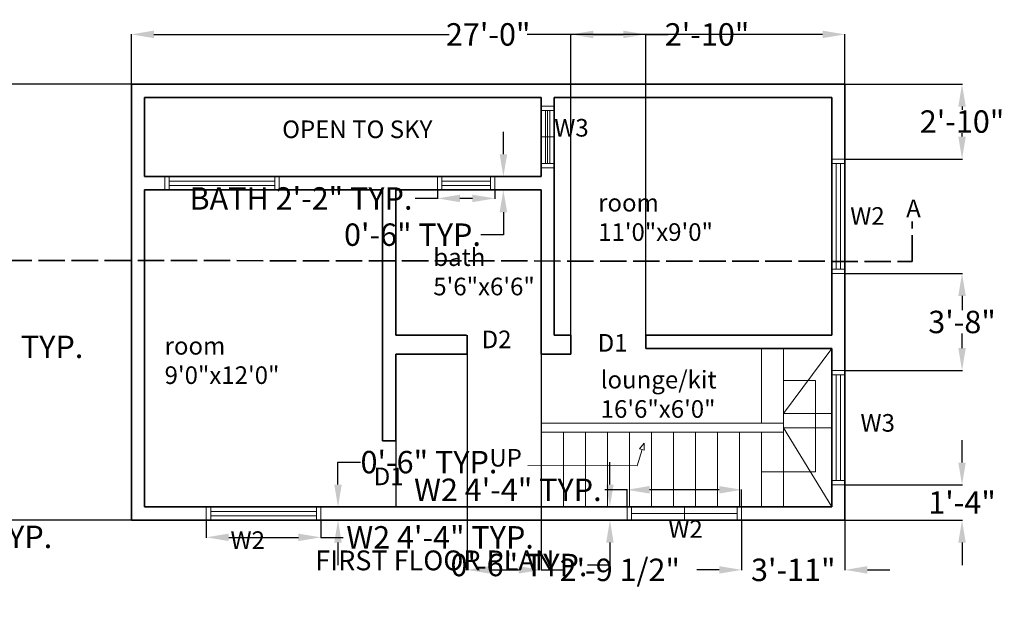
# Model space of a CAD drawing. Units: inches. Extents: x 2393 to 3270, y 740 to 1442.
# Tile 4 of 5: x 2823 to 3270, y 753 to 1018. Entities that reach past the tile are written whole.
import ezdxf

# ---------------------------------------------------------------- set-up
doc = ezdxf.new("R2010")
doc.units = ezdxf.units.IN
doc.header["$MEASUREMENT"] = 0
doc.linetypes.add('ACAD_ISO02W100', pattern=[15, 12, -3])
for name, color, linetype, lineweight in [('A-ANNO-DIMS', 2, 'Continuous', 18), ('A-ANNO-SECT', 1, 'ACAD_ISO02W100', 35), ('A-ANNO-SYMB', 3, 'Continuous', 18), ('A-ANNO-TEXT', 7, 'Continuous', 18), ('A-ANNO-TITL', 7, 'Continuous', 25), ('A-AREA-IDEN', 7, 'Continuous', 18), ('A-DOOR', 3, 'Continuous', 25), ('A-FLOR-STRS', 6, 'Continuous', 18), ('A-GLAZ', 4, 'Continuous', 18), ('A-WALL', 7, 'Continuous', 35)]:
    doc.layers.add(name, color=color, linetype=linetype, lineweight=lineweight)
doc.styles.get("Standard").update_dxf_attribs({"font": 'arial.ttf'})
doc.dimstyles.get("Standard").update_dxf_attribs({"dimtxt": 10.18, "dimasz": 10.18, "dimexe": 0.18, "dimexo": 0.0625, "dimgap": 0.09, "dimtad": 0, "dimtih": 1, "dimtoh": 1, "dimdec": 0, "dimzin": 0, "dimdsep": 46, "dimlunit": 3, "dimtxsty": 'Standard', "dimcen": 0.09, "dimadec": 0, "dimazin": 0, "dimtfac": 1, "dimtdec": 0, "dimtofl": 0, "dimtmove": 0, "dimatfit": 3, "dimfxl": 1, "dimtolj": 1, "dimtzin": 0, "dimarcsym": 0})

# ---------------------------------------------------------------- blocks, each defined once
blk = doc.blocks.new('WIN-52-PLAN')
for p, q in [((0, 6), (0, 0)), ((2, 6), (2, 0)), ((50, 6), (50, 0)), ((52, 6), (52, 0)), ((2, 4), (50, 4)), ((2, 2), (50, 2))]:
    blk.add_line(p, q)
blk = doc.blocks.new('WIN-26-BATH-PLAN')
for p, q in [((0, 0), (0, 6)), ((2, 0), (2, 6)), ((24, 0), (24, 6)), ((26, 0), (26, 6)), ((2, 4), (24, 4)), ((2, 2), (24, 2))]:
    blk.add_line(p, q)
blk = doc.blocks.new('WIN-W3-SIDE-PLAN')
for p, q in [((0, 52), (6, 52)), ((0, 50), (6, 50)), ((2, 50), (2, 2)), ((4, 50), (4, 2)), ((4, 50), (4, 2)), ((4, 50), (4, 2)), ((0, 2), (6, 2)), ((0, 0), (6, 0))]:
    blk.add_line(p, q)
blk = doc.blocks.new('WIN-W2-MULLION-PLAN')
for p, q in [((0, 6), (0, 0)), ((2, 6), (2, 0)), ((26, 6), (26, 0)), ((50, 6), (50, 0)), ((52, 6), (52, 0)), ((2, 3), (50, 3))]:
    blk.add_line(p, q)
blk = doc.blocks.new('WIN-W2-FRONT-PLAN')
for p, q in [((0, 6), (0, 0)), ((2, 6), (2, 0)), ((50, 6), (50, 0)), ((50, 6), (50, 0)), ((52, 6), (52, 0)), ((2, 4), (50, 4)), ((2, 2), (50, 2))]:
    blk.add_line(p, q)
blk = doc.blocks.new('WIN-W3-COURT-PLAN')
for p, q in [((0, 28), (6, 28)), ((0, 26), (6, 26)), ((2, 26), (2, 2)), ((3, 26), (3, 2)), ((4, 26), (4, 2)), ((0, 14), (6, 14)), ((0, 2), (6, 2)), ((0, 0), (6, 0))]:
    blk.add_line(p, q)
blk = doc.blocks.new('STAIR-FLIGHT-PLAN')
for p, q in [((100, 72), (100, 38)), ((100, 72), (100, 38)), ((100, 72), (100, 38)), ((110, 72), (110, 0)), ((110, 72), (110, 0)), ((110, 72), (110, 0)), ((0, 38), (0, 0)), ((110, 38), (0, 38)), ((110, 34), (0, 34)), ((10, 34), (10, 0)), ((20, 34), (20, 0)), ((30, 34), (30, 0)), ((30, 34), (30, 0)), ((30, 34), (30, 0)), ((40, 34), (40, 0)), ((50, 34), (50, 0)), ((60, 34), (60, 0)), ((70, 34), (70, 0)), ((80, 34), (80, 0)), ((80, 34), (80, 0)), ((90, 34), (90, 0)), ((100, 34), (100, 0)), ((100, 34), (100, 0)), ((100, 34), (100, 0))]:
    blk.add_line(p, q)
blk = doc.blocks.new('*D25')
at = {"layer": 'A-ANNO-DIMS', "color": 0, "lineweight": -2, "transparency": 16777216}
for p, q in [((2749.27, 790.69), (2749.27, 782.77)), ((2755.27, 790.69), (2755.27, 782.77)), ((2739.09, 782.95), (2728.91, 782.95)), ((2765.45, 782.95), (2775.63, 782.95))]:
    blk.add_line(p, q, dxfattribs=at)
at = {"layer": 'A-ANNO-DIMS', "color": 0, "transparency": 16777216}
for points in [[(2739.09, 784.65), (2739.09, 781.26), (2749.27, 782.95)], [(2765.45, 784.65), (2765.45, 781.26), (2755.27, 782.95)]]:
    blk.add_solid(points, dxfattribs=at)
at = {"layer": 'Defpoints', "color": 0, "transparency": 16777216}
for p in [(2749.27, 790.75), (2755.27, 790.75), (2755.27, 782.95)]:
    blk.add_point(p, dxfattribs=at)
at = {"layer": 'A-ANNO-DIMS', "color": 0, "transparency": 16777216, "insert": (2806.75, 782.95), "char_height": 10.18, "attachment_point": 5}
blk.add_mtext('\\A1;0\'-6" TYP.', dxfattribs=at)
blk = doc.blocks.new('*D26')
at = {"layer": 'A-ANNO-DIMS', "color": 0, "lineweight": -2, "transparency": 16777216}
for p, q in [((3098.85, 804.33), (3088.67, 804.33)), ((3098.85, 796.6), (3098.85, 804.51)), ((3140.67, 804.33), (3109.03, 804.33)), ((3150.85, 796.6), (3150.85, 804.51))]:
    blk.add_line(p, q, dxfattribs=at)
at = {"layer": 'A-ANNO-DIMS', "color": 0, "transparency": 16777216}
for points in [[(3109.03, 806.03), (3109.03, 802.64), (3098.85, 804.33)], [(3140.67, 806.03), (3140.67, 802.64), (3150.85, 804.33)]]:
    blk.add_solid(points, dxfattribs=at)
at = {"layer": 'Defpoints', "color": 0, "transparency": 16777216}
for p in [(3098.85, 804.33), (3098.85, 796.53), (3150.85, 796.53)]:
    blk.add_point(p, dxfattribs=at)
at = {"layer": 'A-ANNO-DIMS', "color": 0, "transparency": 16777216, "insert": (3044.7, 804.33), "char_height": 10.18, "attachment_point": 5}
blk.add_mtext('\\A1;W2 4\'-4" TYP.', dxfattribs=at)
blk = doc.blocks.new('*D27')
at = {"layer": 'A-ANNO-DIMS', "color": 0, "lineweight": -2, "transparency": 16777216}
for p, q in [((3091.05, 806.71), (3091.05, 816.89)), ((3098.78, 796.53), (3090.87, 796.53)), ((3098.78, 790.53), (3090.87, 790.53)), ((3091.05, 780.35), (3091.05, 770.17)), ((3091.05, 770.17), (3080.87, 770.17))]:
    blk.add_line(p, q, dxfattribs=at)
at = {"layer": 'A-ANNO-DIMS', "color": 0, "transparency": 16777216}
for points in [[(3089.35, 806.71), (3092.74, 806.71), (3091.05, 796.53)], [(3089.35, 780.35), (3092.74, 780.35), (3091.05, 790.53)]]:
    blk.add_solid(points, dxfattribs=at)
at = {"layer": 'Defpoints', "color": 0, "transparency": 16777216}
for p in [(3098.85, 796.53), (3091.05, 790.53), (3098.85, 790.53)]:
    blk.add_point(p, dxfattribs=at)
at = {"layer": 'A-ANNO-DIMS', "color": 0, "transparency": 16777216, "insert": (3049.75, 770.17), "char_height": 10.18, "attachment_point": 5}
blk.add_mtext('\\A1;0\'-6" TYP.', dxfattribs=at)
blk = doc.blocks.new('*D28')
at = {"layer": 'A-ANNO-DIMS', "color": 0, "lineweight": -2, "transparency": 16777216}
for p, q in [((3012.78, 940.47), (3012.78, 936.45)), ((3038.78, 940.47), (3038.78, 936.45)), ((3012.78, 936.63), (3002.6, 936.63)), ((3028.6, 936.63), (3022.96, 936.63))]:
    blk.add_line(p, q, dxfattribs=at)
at = {"layer": 'A-ANNO-DIMS', "color": 0, "transparency": 16777216}
for points in [[(3022.96, 938.33), (3022.96, 934.94), (3012.78, 936.63)], [(3028.6, 938.33), (3028.6, 934.94), (3038.78, 936.63)]]:
    blk.add_solid(points, dxfattribs=at)
at = {"layer": 'Defpoints', "color": 0, "transparency": 16777216}
for p in [(3012.78, 940.53), (3038.78, 940.53), (3012.78, 936.63)]:
    blk.add_point(p, dxfattribs=at)
at = {"layer": 'A-ANNO-DIMS', "color": 0, "transparency": 16777216, "insert": (2950.77, 936.63), "char_height": 10.18, "attachment_point": 5}
blk.add_mtext('\\A1;BATH 2\'-2" TYP.', dxfattribs=at)
blk = doc.blocks.new('*D29')
at = {"layer": 'A-ANNO-DIMS', "color": 0, "lineweight": -2, "transparency": 16777216}
for p, q in [((3042.68, 956.71), (3042.68, 966.89)), ((3038.84, 946.53), (3042.86, 946.53)), ((3038.84, 940.53), (3042.86, 940.53)), ((3042.68, 930.35), (3042.68, 920.17)), ((3042.68, 920.17), (3032.5, 920.17))]:
    blk.add_line(p, q, dxfattribs=at)
at = {"layer": 'A-ANNO-DIMS', "color": 0, "transparency": 16777216}
for points in [[(3040.98, 956.71), (3044.38, 956.71), (3042.68, 946.53)], [(3040.98, 930.35), (3044.38, 930.35), (3042.68, 940.53)]]:
    blk.add_solid(points, dxfattribs=at)
at = {"layer": 'Defpoints', "color": 0, "transparency": 16777216}
for p in [(3038.78, 946.53), (3038.78, 940.53), (3042.68, 940.53)]:
    blk.add_point(p, dxfattribs=at)
at = {"layer": 'A-ANNO-DIMS', "color": 0, "transparency": 16777216, "insert": (3001.39, 920.17), "char_height": 10.18, "attachment_point": 5}
blk.add_mtext('\\A1;0\'-6" TYP.', dxfattribs=at)
blk = doc.blocks.new('*D30')
at = {"layer": 'A-ANNO-DIMS', "color": 0, "lineweight": -2, "transparency": 16777216}
for p, q in [((2907.78, 790.47), (2907.78, 782.55)), ((2959.78, 790.47), (2959.78, 782.55)), ((2917.96, 782.73), (2949.6, 782.73)), ((2959.78, 782.73), (2969.96, 782.73))]:
    blk.add_line(p, q, dxfattribs=at)
at = {"layer": 'A-ANNO-DIMS', "color": 0, "transparency": 16777216}
for points in [[(2917.96, 784.43), (2917.96, 781.04), (2907.78, 782.73)], [(2949.6, 784.43), (2949.6, 781.04), (2959.78, 782.73)]]:
    blk.add_solid(points, dxfattribs=at)
at = {"layer": 'Defpoints', "color": 0, "transparency": 16777216}
for p in [(2907.78, 790.53), (2959.78, 790.53), (2959.78, 782.73)]:
    blk.add_point(p, dxfattribs=at)
at = {"layer": 'A-ANNO-DIMS', "color": 0, "transparency": 16777216, "insert": (3013.93, 782.73), "char_height": 10.18, "attachment_point": 5}
blk.add_mtext('\\A1;W2 4\'-4" TYP.', dxfattribs=at)
blk = doc.blocks.new('*D31')
at = {"layer": 'A-ANNO-DIMS', "color": 0, "lineweight": -2, "transparency": 16777216}
for p, q in [((2967.58, 806.71), (2967.58, 816.89)), ((2967.58, 816.89), (2977.76, 816.89)), ((2959.84, 796.53), (2967.76, 796.53)), ((2959.84, 790.53), (2967.76, 790.53)), ((2967.58, 780.35), (2967.58, 770.17))]:
    blk.add_line(p, q, dxfattribs=at)
at = {"layer": 'A-ANNO-DIMS', "color": 0, "transparency": 16777216}
for points in [[(2965.88, 806.71), (2969.28, 806.71), (2967.58, 796.53)], [(2965.88, 780.35), (2969.28, 780.35), (2967.58, 790.53)]]:
    blk.add_solid(points, dxfattribs=at)
at = {"layer": 'Defpoints', "color": 0, "transparency": 16777216}
for p in [(2959.78, 796.53), (2967.58, 796.53), (2959.78, 790.53)]:
    blk.add_point(p, dxfattribs=at)
at = {"layer": 'A-ANNO-DIMS', "color": 0, "transparency": 16777216, "insert": (3008.88, 816.89), "char_height": 10.18, "attachment_point": 5}
blk.add_mtext('\\A1;0\'-6" TYP.', dxfattribs=at)
blk = doc.blocks.new('*D34')
at = {"layer": 'A-ANNO-DIMS', "color": 0, "lineweight": -2, "transparency": 16777216}
for p, q in [((2617.41, 852.81), (2617.41, 869.43)), ((2627.59, 869.25), (2717.23, 869.25)), ((2727.41, 852.81), (2727.41, 869.43)), ((2727.41, 869.25), (2737.59, 869.25))]:
    blk.add_line(p, q, dxfattribs=at)
at = {"layer": 'A-ANNO-DIMS', "color": 0, "transparency": 16777216}
for points in [[(2627.59, 870.95), (2627.59, 867.56), (2617.41, 869.25)], [(2717.23, 870.95), (2717.23, 867.56), (2727.41, 869.25)]]:
    blk.add_solid(points, dxfattribs=at)
at = {"layer": 'Defpoints', "color": 0, "transparency": 16777216}
for p in [(2727.41, 869.25), (2617.41, 852.75), (2727.41, 852.75)]:
    blk.add_point(p, dxfattribs=at)
at = {"layer": 'A-ANNO-DIMS', "color": 0, "transparency": 16777216, "insert": (2795.67, 869.25), "char_height": 10.18, "attachment_point": 5}
blk.add_mtext('\\A1;FLIGHT 9\'-2" TYP.', dxfattribs=at)
blk = doc.blocks.new('*D49')
at = {"layer": 'A-ANNO-DIMS', "color": 0, "lineweight": -2, "transparency": 16777216}
for p, q in [((3250.94, 816.71), (3250.94, 826.89)), ((3197.84, 806.53), (3251.12, 806.53)), ((3197.84, 790.53), (3251.12, 790.53)), ((3250.94, 780.35), (3250.94, 770.17))]:
    blk.add_line(p, q, dxfattribs=at)
at = {"layer": 'A-ANNO-DIMS', "color": 0, "transparency": 16777216}
for points in [[(3249.24, 816.71), (3252.64, 816.71), (3250.94, 806.53)], [(3249.24, 780.35), (3252.64, 780.35), (3250.94, 790.53)]]:
    blk.add_solid(points, dxfattribs=at)
at = {"layer": 'Defpoints', "color": 0, "transparency": 16777216}
for p in [(3197.78, 806.53), (3250.94, 806.53), (3197.78, 790.53)]:
    blk.add_point(p, dxfattribs=at)
at = {"layer": 'A-ANNO-DIMS', "color": 0, "transparency": 16777216, "insert": (3250.94, 798.53), "char_height": 10.18, "attachment_point": 5}
blk.add_mtext('\\A1;1\'-4"', dxfattribs=at)
blk = doc.blocks.new('*D50')
at = {"layer": 'A-ANNO-DIMS', "color": 0, "lineweight": -2, "transparency": 16777216}
for p, q in [((3197.84, 902.53), (3251.12, 902.53)), ((3250.94, 892.35), (3250.94, 885.83)), ((3250.94, 868.71), (3250.94, 875.24)), ((3197.84, 858.53), (3251.12, 858.53))]:
    blk.add_line(p, q, dxfattribs=at)
at = {"layer": 'A-ANNO-DIMS', "color": 0, "transparency": 16777216}
for points in [[(3249.24, 892.35), (3252.64, 892.35), (3250.94, 902.53)], [(3249.24, 868.71), (3252.64, 868.71), (3250.94, 858.53)]]:
    blk.add_solid(points, dxfattribs=at)
at = {"layer": 'Defpoints', "color": 0, "transparency": 16777216}
for p in [(3197.78, 902.53), (3250.94, 902.53), (3197.78, 858.53)]:
    blk.add_point(p, dxfattribs=at)
at = {"layer": 'A-ANNO-DIMS', "color": 0, "transparency": 16777216, "insert": (3250.94, 880.53), "char_height": 10.18, "attachment_point": 5}
blk.add_mtext('\\A1;3\'-8"', dxfattribs=at)
blk = doc.blocks.new('*D51')
at = {"layer": 'A-ANNO-DIMS', "color": 0, "lineweight": -2, "transparency": 16777216}
for p, q in [((3197.84, 988.53), (3251.12, 988.53)), ((3250.94, 978.35), (3250.94, 976.82)), ((3250.94, 964.71), (3250.94, 966.25)), ((3197.84, 954.53), (3251.12, 954.53))]:
    blk.add_line(p, q, dxfattribs=at)
at = {"layer": 'A-ANNO-DIMS', "color": 0, "transparency": 16777216}
for points in [[(3249.24, 978.35), (3252.64, 978.35), (3250.94, 988.53)], [(3249.24, 964.71), (3252.64, 964.71), (3250.94, 954.53)]]:
    blk.add_solid(points, dxfattribs=at)
at = {"layer": 'Defpoints', "color": 0, "transparency": 16777216}
for p in [(3197.78, 988.53), (3250.94, 988.53), (3197.78, 954.53)]:
    blk.add_point(p, dxfattribs=at)
at = {"layer": 'A-ANNO-DIMS', "color": 0, "transparency": 16777216, "insert": (3250.94, 971.53), "char_height": 10.18, "attachment_point": 5}
blk.add_mtext('\\A1;2\'-10"', dxfattribs=at)
blk = doc.blocks.new('*D52')
at = {"layer": 'A-ANNO-DIMS', "color": 0, "lineweight": -2, "transparency": 16777216}
for p, q in [((3150.85, 790.47), (3150.85, 767.78)), ((3197.78, 790.47), (3197.78, 767.78)), ((3140.67, 767.96), (3130.49, 767.96)), ((3207.96, 767.96), (3218.14, 767.96))]:
    blk.add_line(p, q, dxfattribs=at)
at = {"layer": 'A-ANNO-DIMS', "color": 0, "transparency": 16777216}
for points in [[(3140.67, 769.66), (3140.67, 766.26), (3150.85, 767.96)], [(3207.96, 769.66), (3207.96, 766.26), (3197.78, 767.96)]]:
    blk.add_solid(points, dxfattribs=at)
at = {"layer": 'Defpoints', "color": 0, "transparency": 16777216}
for p in [(3150.85, 790.53), (3197.78, 790.53), (3197.78, 767.96)]:
    blk.add_point(p, dxfattribs=at)
at = {"layer": 'A-ANNO-DIMS', "color": 0, "transparency": 16777216, "insert": (3174.31, 767.96), "char_height": 10.18, "attachment_point": 5}
blk.add_mtext('\\A1;3\'-11"', dxfattribs=at)
blk = doc.blocks.new('*D53')
at = {"layer": 'A-ANNO-DIMS', "color": 0, "lineweight": -2, "transparency": 16777216}
for p, q in [((2873.78, 988.6), (2873.78, 1011.29)), ((2883.96, 1011.11), (3018.12, 1011.11)), ((3187.6, 1011.11), (3053.44, 1011.11)), ((3197.78, 988.6), (3197.78, 1011.29))]:
    blk.add_line(p, q, dxfattribs=at)
at = {"layer": 'A-ANNO-DIMS', "color": 0, "transparency": 16777216}
for points in [[(2883.96, 1012.81), (2883.96, 1009.41), (2873.78, 1011.11)], [(3187.6, 1012.81), (3187.6, 1009.41), (3197.78, 1011.11)]]:
    blk.add_solid(points, dxfattribs=at)
at = {"layer": 'Defpoints', "color": 0, "transparency": 16777216}
for p in [(3197.78, 1011.11), (2873.78, 988.53), (3197.78, 988.53)]:
    blk.add_point(p, dxfattribs=at)
at = {"layer": 'A-ANNO-DIMS', "color": 0, "transparency": 16777216, "insert": (3035.78, 1011.11), "char_height": 10.18, "attachment_point": 5}
blk.add_mtext('\\A1;27\'-0"', dxfattribs=at)
blk = doc.blocks.new('*D54')
at = {"layer": 'A-ANNO-DIMS', "color": 0, "lineweight": -2, "transparency": 16777216}
for p, q in [((2873.72, 988.53), (2763.87, 988.53)), ((2764.05, 978.35), (2764.05, 894.82)), ((2764.05, 800.71), (2764.05, 884.25)), ((2873.72, 790.53), (2763.87, 790.53))]:
    blk.add_line(p, q, dxfattribs=at)
at = {"layer": 'A-ANNO-DIMS', "color": 0, "transparency": 16777216}
for points in [[(2762.35, 978.35), (2765.75, 978.35), (2764.05, 988.53)], [(2762.35, 800.71), (2765.75, 800.71), (2764.05, 790.53)]]:
    blk.add_solid(points, dxfattribs=at)
at = {"layer": 'Defpoints', "color": 0, "transparency": 16777216}
for p in [(2764.05, 988.53), (2873.78, 988.53), (2873.78, 790.53)]:
    blk.add_point(p, dxfattribs=at)
at = {"layer": 'A-ANNO-DIMS', "color": 0, "transparency": 16777216, "insert": (2764.05, 889.53), "char_height": 10.18, "attachment_point": 5}
blk.add_mtext('\\A1;16\'-6"', dxfattribs=at)
blk = doc.blocks.new('*D55')
at = {"layer": 'A-ANNO-DIMS', "color": 0, "lineweight": -2, "transparency": 16777216}
for p, q in [((3026.23, 865.83), (3026.23, 767.78)), ((3059.78, 865.83), (3059.78, 767.78)), ((3036.41, 767.96), (3049.6, 767.96)), ((3059.78, 767.96), (3069.96, 767.96))]:
    blk.add_line(p, q, dxfattribs=at)
at = {"layer": 'A-ANNO-DIMS', "color": 0, "transparency": 16777216}
for points in [[(3036.41, 769.66), (3036.41, 766.26), (3026.23, 767.96)], [(3049.6, 769.66), (3049.6, 766.26), (3059.78, 767.96)]]:
    blk.add_solid(points, dxfattribs=at)
at = {"layer": 'Defpoints', "color": 0, "transparency": 16777216}
for p in [(3026.23, 865.89), (3059.78, 865.89), (3059.78, 767.96)]:
    blk.add_point(p, dxfattribs=at)
at = {"layer": 'A-ANNO-DIMS', "color": 0, "transparency": 16777216, "insert": (3095.53, 767.96), "char_height": 10.18, "attachment_point": 5}
blk.add_mtext('\\A1;2\'-9 1/2"', dxfattribs=at)
blk = doc.blocks.new('*D56')
at = {"layer": 'A-ANNO-DIMS', "color": 0, "lineweight": -2, "transparency": 16777216}
for p, q in [((3073.35, 874.6), (3073.35, 1011.29)), ((3083.53, 1011.11), (3097.13, 1011.11)), ((3107.31, 874.6), (3107.31, 1011.29)), ((3107.31, 1011.11), (3117.49, 1011.11))]:
    blk.add_line(p, q, dxfattribs=at)
at = {"layer": 'A-ANNO-DIMS', "color": 0, "transparency": 16777216}
for points in [[(3083.53, 1012.81), (3083.53, 1009.41), (3073.35, 1011.11)], [(3097.13, 1012.81), (3097.13, 1009.41), (3107.31, 1011.11)]]:
    blk.add_solid(points, dxfattribs=at)
at = {"layer": 'Defpoints', "color": 0, "transparency": 16777216}
for p in [(3107.31, 1011.11), (3073.35, 874.53), (3107.31, 874.53)]:
    blk.add_point(p, dxfattribs=at)
at = {"layer": 'A-ANNO-DIMS', "color": 0, "transparency": 16777216, "insert": (3135.15, 1011.11), "char_height": 10.18, "attachment_point": 5}
blk.add_mtext('\\A1;2\'-10"', dxfattribs=at)

msp = doc.modelspace()

# ---------------------------------------------------------------- linework, layer by layer
at = {"layer": 'A-ANNO-SECT'}
for p, q in [((3228.37, 908.02), (3228.37, 926.08)), ((2786.62, 908.53), (3228.37, 908.02))]:
    msp.add_line(p, q, dxfattribs=at)
at = {"layer": 'A-ANNO-SYMB'}
for p, q in [((3106.64, 825.49), (3104.48, 822.93)), ((3105.75, 822.55), (3104.48, 822.93)), ((3104.48, 822.93), (3106.64, 822.28)), ((3106.64, 822.28), (3106.64, 825.49)), ((3103.48, 815.13), (3105.75, 822.55)), ((3053.71, 815.38), (3103.48, 815.13))]:
    msp.add_line(p, q, dxfattribs=at)
at = {"layer": 'A-DOOR'}
msp.add_line((2993.78, 826.53), (2993.78, 796.53), dxfattribs=at)
at = {"layer": 'A-FLOR-STRS'}
for p, q in [((3169.92, 838.97), (3191.78, 868.53)), ((3169.92, 853.88), (3169.92, 853.88)), ((3169.92, 853.88), (3184.39, 853.88)), ((3184.39, 853.88), (3184.39, 812.49)), ((3169.92, 838.97), (3191.78, 838.97)), ((3169.92, 832.53), (3191.78, 832.53)), ((3169.92, 832.53), (3191.78, 796.53)), ((3184.39, 812.49), (3159.92, 812.49))]:
    msp.add_line(p, q, dxfattribs=at)
at = {"layer": 'A-WALL'}
for p, q in [((2873.78, 790.53), (2873.78, 988.53)), ((2873.78, 988.53), (3197.78, 988.53)), ((3197.78, 988.53), (3197.78, 790.53)), ((2879.78, 946.53), (2879.78, 982.53)), ((2879.78, 982.53), (2987.78, 982.53)), ((2987.78, 982.53), (2993.78, 982.53)), ((2993.78, 982.53), (3059.78, 982.53)), ((3059.78, 946.53), (3059.78, 982.53)), ((3065.78, 874.53), (3065.78, 982.53)), ((3065.78, 982.53), (3191.78, 982.53)), ((3191.78, 982.53), (3191.78, 874.53)), ((2987.78, 946.53), (2879.78, 946.53)), ((2993.78, 946.53), (2987.78, 946.53)), ((3059.78, 946.53), (2993.78, 946.53)), ((2879.78, 862.53), (2879.78, 940.53)), ((2987.78, 940.53), (2879.78, 940.53)), ((2987.78, 862.53), (2987.78, 940.53)), ((2993.78, 874.53), (2993.78, 940.53)), ((3059.78, 940.53), (2993.78, 940.53)), ((3059.78, 940.53), (3059.78, 865.89)), ((2993.78, 874.53), (3025.95, 874.53)), ((3026.23, 865.89), (3026.23, 874.53)), ((3065.78, 874.53), (3073.35, 874.53)), ((3073.35, 874.53), (3073.35, 868.53)), ((3107.31, 874.53), (3191.78, 874.53)), ((3107.31, 874.53), (3107.31, 868.53)), ((3073.35, 865.89), (3073.35, 868.53)), ((3107.31, 868.53), (3191.78, 868.53)), ((3191.78, 868.53), (3191.78, 796.53)), ((2993.78, 862.53), (2993.78, 865.89)), ((2993.78, 865.89), (3026.23, 865.89)), ((3059.78, 865.89), (3065.78, 865.89)), ((3065.78, 865.89), (3073.35, 865.89)), ((2879.78, 856.53), (2879.78, 862.53)), ((2987.78, 856.53), (2987.78, 862.53)), ((2993.78, 862.53), (2993.78, 856.53)), ((2879.78, 796.53), (2879.78, 856.53)), ((2987.78, 826.53), (2987.78, 856.53)), ((2993.78, 826.53), (2993.78, 856.53)), ((2987.78, 826.53), (2993.78, 826.53)), ((2987.78, 796.53), (2879.78, 796.53)), ((2987.78, 796.53), (2993.78, 796.53)), ((3011.44, 796.53), (2993.78, 796.53)), ((3011.44, 796.53), (3057.91, 796.53)), ((3191.78, 796.53), (3057.91, 796.53)), ((3011.44, 790.53), (2873.78, 790.53)), ((3011.44, 790.53), (3057.91, 790.53)), ((3197.78, 790.53), (3057.91, 790.53))]:
    msp.add_line(p, q, dxfattribs=at)

# ---------------------------------------------------------------- block references
at = {"layer": 'A-FLOR-STRS'}
msp.add_blockref('STAIR-FLIGHT-PLAN', (3059.92, 796.53), dxfattribs=at)
at = {"layer": 'A-GLAZ'}
for name, p, rotation in [('WIN-W3-COURT-PLAN', (3065.78, 978.53), 180), ('WIN-52-PLAN', (3191.78, 954.53), 269.9999999999983), ('WIN-52-PLAN', (2940.92, 946.53), 180), ('WIN-26-BATH-PLAN', (3038.78, 946.53), 180), ('WIN-W2-MULLION-PLAN', (3150.85, 796.53), 180)]:
    msp.add_blockref(name, p, dxfattribs=dict(at, rotation=rotation))
for name, p in [('WIN-W3-SIDE-PLAN', (3191.78, 806.53)), ('WIN-W2-FRONT-PLAN', (2907.78, 790.53))]:
    msp.add_blockref(name, p, dxfattribs=at)

# ---------------------------------------------------------------- texts
at = {"layer": 'A-ANNO-SYMB', "char_height": 8, "attachment_point": 1}
for s, insert in [('A', (3225.57, 936.1)), ('UP', (3036.3, 822.87))]:
    msp.add_mtext_dynamic_manual_height_columns(s, width=76.737, gutter_width=1, heights=[0], dxfattribs=dict(at, insert=insert))
at = {"layer": 'A-ANNO-TEXT', "char_height": 8, "attachment_point": 1}
for s, insert in [('W3', (3065.78, 972.71)), ('W2', (3200.17, 932.66)), ('D2', (3032.8, 876.61)), ('D1', (3085.51, 875.05)), ('W3', (3204.82, 838.71)), ('D1', (2983.81, 814.41)), ('W2', (3117.58, 790.52)), ('W2', (2918.77, 785.46))]:
    msp.add_mtext_dynamic_manual_height_columns(s, width=76.737, gutter_width=1, heights=[0], dxfattribs=dict(at, insert=insert))
at = {"layer": 'A-ANNO-TITL', "insert": (2957.26, 776.76), "char_height": 9, "attachment_point": 1}
msp.add_mtext_dynamic_manual_height_columns('FIRST FLOOR PLAN', width=140.3126, gutter_width=1, heights=[0], dxfattribs=at)
at = {"layer": 'A-AREA-IDEN', "char_height": 8, "attachment_point": 1}
for s, insert in [('OPEN TO SKY', (2942.23, 972.02)), ('room\\P11\'0"x9\'0"', (3085.7, 938.69)), ('bath\\P5\'6"x6\'6"', (3010.85, 913.96)), ('room\\P9\'0"x12\'0"', (2888.85, 873.71)), ('lounge/kit\\P16\'6"x6\'0"', (3086.86, 858.34))]:
    msp.add_mtext_dynamic_manual_height_columns(s, width=76.737, gutter_width=1, heights=[0], dxfattribs=dict(at, insert=insert))

# ---------------------------------------------------------------- dimensions: what is measured, and where the dimension line sits
at = {"layer": 'A-ANNO-DIMS'}
for base, p1, p2, picture, middle in [((3197.78, 1011.11), (2873.78, 988.53), (3197.78, 988.53), '*D53', (3035.78, 1011.11)), ((3107.31, 1011.11), (3073.35, 874.53), (3107.31, 874.53), '*D56', (3135.15, 1011.11)), ((3059.7813, 767.9593), (3026.2264, 865.893), (3059.7813, 865.893), '*D55', (3095.5291, 767.9593)), ((3197.78, 767.96), (3150.85, 790.53), (3197.78, 790.53), '*D52', (3174.31, 767.96))]:
    dim = msp.add_linear_dim(base=base, p1=p1, p2=p2, dimstyle='Standard', override={"dimdec": 1, "dimlfac": 1, "dimrnd": 0, "dimzin": 1, "dimdsep": 46, "dimlunit": 4, "dimfrac": 2}, dxfattribs=at)
    dim.commit()
    dim.dimension.update_dxf_attribs({"geometry": picture, "text_midpoint": middle})
for base, p1, p2, picture, middle in [((2764.05, 988.53), (2873.78, 790.53), (2873.78, 988.53), '*D54', (2764.05, 889.53)), ((3250.94, 988.53), (3197.78, 954.53), (3197.78, 988.53), '*D51', (3250.94, 971.53)), ((3250.94, 902.53), (3197.78, 858.53), (3197.78, 902.53), '*D50', (3250.94, 880.53)), ((3250.94, 806.53), (3197.78, 790.53), (3197.78, 806.53), '*D49', (3250.94, 798.53))]:
    dim = msp.add_linear_dim(base=base, p1=p1, p2=p2, angle=90, dimstyle='Standard', override={"dimdec": 1, "dimlfac": 1, "dimrnd": 0, "dimzin": 1, "dimdsep": 46, "dimlunit": 4, "dimfrac": 2}, dxfattribs=at)
    dim.commit()
    dim.dimension.update_dxf_attribs({"geometry": picture, "text_midpoint": middle})
for base, p1, p2, angle, text, picture, middle in [((3042.68, 940.53), (3038.78, 946.53), (3038.78, 940.53), 270, '<> TYP.', '*D29', (3001.39, 920.17)), ((3012.78, 936.63), (3038.78, 940.53), (3012.78, 940.53), 180, 'BATH <> TYP.', '*D28', (2950.77, 936.63)), ((2967.58, 796.53), (2959.78, 790.53), (2959.78, 796.53), 90, '<> TYP.', '*D31', (3008.88, 816.89)), ((3098.85, 804.33), (3150.85, 796.53), (3098.85, 796.53), 180, 'W2 <> TYP.', '*D26', (3044.7, 804.33)), ((3091.05, 790.53), (3098.85, 796.53), (3098.85, 790.53), 270, '<> TYP.', '*D27', (3049.75, 770.17))]:
    dim = msp.add_linear_dim(base=base, p1=p1, p2=p2, angle=angle, text=text, dimstyle='Standard', override={"dimdec": 1, "dimlfac": 1, "dimrnd": 0, "dimzin": 1, "dimdsep": 46, "dimlunit": 4, "dimfrac": 2}, dxfattribs=at)
    dim.commit()
    dim.dimension.update_dxf_attribs({"geometry": picture, "text_midpoint": middle})
for base, p1, p2, text, picture, middle in [((2727.41, 869.25), (2617.41, 852.75), (2727.41, 852.75), 'FLIGHT <> TYP.', '*D34', (2795.67, 869.25)), ((2959.78, 782.73), (2907.78, 790.53), (2959.78, 790.53), 'W2 <> TYP.', '*D30', (3013.93, 782.73)), ((2755.27, 782.95), (2749.27, 790.75), (2755.27, 790.75), '<> TYP.', '*D25', (2806.75, 782.95))]:
    dim = msp.add_linear_dim(base=base, p1=p1, p2=p2, text=text, dimstyle='Standard', override={"dimdec": 1, "dimlfac": 1, "dimrnd": 0, "dimzin": 1, "dimdsep": 46, "dimlunit": 4, "dimfrac": 2}, dxfattribs=at)
    dim.commit()
    dim.dimension.update_dxf_attribs({"geometry": picture, "text_midpoint": middle})

doc.saveas('drawing.dxf')
